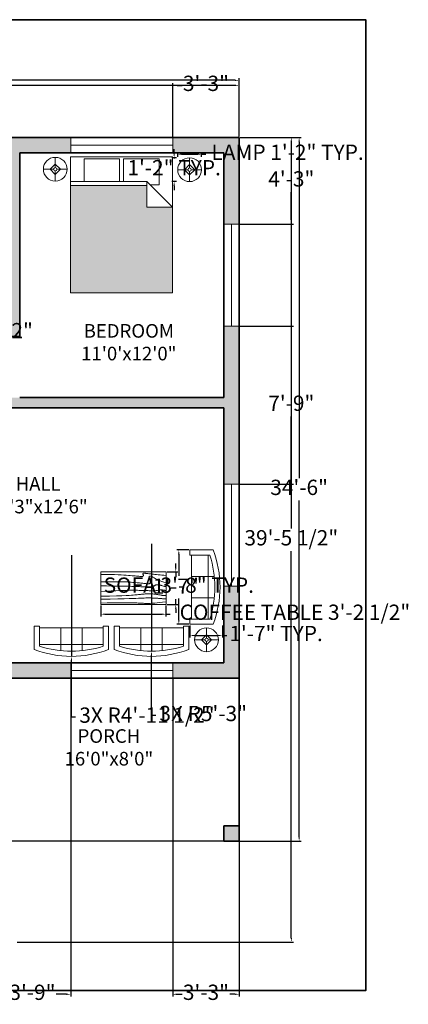
# Model space of a CAD drawing. Units: inches. Extents: x 1329 to 1989, y 1493 to 2072.
# Tile 4 of 4: x 1761 to 1989, y 1493 to 2072. Entities that reach past the tile are written whole.
import ezdxf

# ---------------------------------------------------------------- set-up
doc = ezdxf.new("R2010")
doc.units = ezdxf.units.IN
for name, color, linetype, lineweight in [('A-ANNO-DIMS', 2, 'Continuous', 18), ('A-ANNO-TTLB', 7, 'Continuous', 35), ('A-AREA-IDEN', 7, 'Continuous', 25), ('A-COLS', 7, 'Continuous', 35), ('A-FLOR', 7, 'Continuous', 25), ('A-FURN', 8, 'Continuous', 18), ('A-GLAZ', 4, 'Continuous', 18), ('A-WALL', 7, 'Continuous', 35)]:
    doc.layers.add(name, color=color, linetype=linetype, lineweight=lineweight)
for name, color, linetype, lineweight, true_color in [('A-COLS-PATT', 251, 'Continuous', 13, 0x636466), ('A-FURN-PATT', 18, 'Continuous', 13, 0x000000), ('A-WALL-PATT', 251, 'Continuous', 13, 0x636466)]:
    doc.layers.add(name, color=color, linetype=linetype, lineweight=lineweight, true_color=true_color)
doc.styles.get("Standard").update_dxf_attribs({"font": 'arial.ttf'})
doc.dimstyles.new('ISO-25', dxfattribs={"dimtxt": 9, "dimasz": 2.5, "dimexe": 1.25, "dimexo": 0.625, "dimgap": 2, "dimtad": 0, "dimtih": 1, "dimtoh": 1, "dimdec": 1, "dimlunit": 4, "dimtxsty": 'Standard', "dimcen": 2.5, "dimadec": 0, "dimazin": 0, "dimtfac": 0.5, "dimtdec": 1, "dimtmove": 0, "dimatfit": 3, "dimfxl": 1, "dimarcsym": 0})

# ---------------------------------------------------------------- blocks, each defined once
blk = doc.blocks.new('Bed - Queen')
for p, q in [((0, -80.00003), (0, 0)), ((0, 0), (59.99999, 0)), ((59.99999, 0), (59.99999, -80.00003)), ((7.99999, -1.2), (28.79998, -1.2)), ((7.99999, -14.4), (7.99999, -1.2)), ((28.79998, -1.2), (28.79998, -14.4)), ((31.19999, -1.2), (51.99999, -1.2)), ((31.19999, -14.4), (31.19999, -1.2)), ((51.99999, -1.2), (51.99999, -16.4)), ((0, -14.4), (44.8, -14.4)), ((44.8, -16.8), (0, -16.8)), ((59.99999, -29.6), (44.8, -14.4)), ((44.8, -14.4), (44.8, -29.6)), ((51.99999, -16.4), (46.79936, -16.4)), ((44.8, -29.6), (59.99999, -29.6)), ((59.99999, -80.00003), (0, -80.00003))]:
    blk.add_line(p, q)
blk = doc.blocks.new('Lamp - Table')
for p, q in [((0, 7), (0, 1)), ((-1, 0), (-7, 0)), ((0, 3), (-3, 0)), ((-3, 0), (0, -3)), ((3, 0), (0, 3)), ((0, -3), (3, 0)), ((1, 0), (7, 0)), ((0, -1), (0, -7))]:
    blk.add_line(p, q)
for radius in [7, 1]:
    blk.add_circle((0, 0), radius)
blk = doc.blocks.new('Sofa - Roundback 7 ft.')
for p, q in [((-12.00002, -32.4421), (-12.00003, -6.5971)), ((11.99997, -32.4421), (11.99998, -6.5971)), ((-36.000027, -34), (-36.000027, -11.4696)), ((-35.999844, -13.3819), (35.9998, -13.3819)), ((35.99998, -34), (35.99998, -11.4696)), ((-36.000027, -32.4421), (35.99998, -32.4421))]:
    blk.add_line(p, q)
for points in [[(-36.000027, -34), (-42.000027, -34), (-42.000027, -8)], [(41.99998, -8), (41.99998, -34), (35.99998, -34)]]:
    blk.add_lwpolyline(points)
for centre, radius, start, end in [((0, -114.25), 114.25, 68.43141, 111.5686), ((-0.00001, -127.1968), 121.1968, 72.72033, 107.2797)]:
    blk.add_arc(centre, radius, start, end)
blk = doc.blocks.new('Table - Rectangular Woodgrain 60 x 30 in.')
for p, q in [((0, 0), (0, -30)), ((60, 0), (0, 0)), ((60, -30), (60, 0)), ((0, -30), (60, -30))]:
    blk.add_line(p, q)
for points in [[(0, -2.4), (4.8155, -2.418), (9.0302, -2.4688), (12.709, -2.5477), (15.9167, -2.65), (18.7181, -2.7711), (21.1781, -2.9063), (23.3616, -3.0508), (25.3333, -3.2), (27.1477, -3.3495), (28.8172, -3.4958), (30.3437, -3.636), (31.7291, -3.7667), (32.9756, -3.8849), (34.0849, -3.9875), (35.059, -4.0714), (35.9, -4.1334), (36.6114, -4.1711), (37.2041, -4.1854), (37.6906, -4.1779), (38.0833, -4.15), (38.3948, -4.1034), (38.6375, -4.0396), (38.8239, -3.9602), (38.9666, -3.8667), (39.0764, -3.7608), (39.1573, -3.6448), (39.2116, -3.521), (39.2416, -3.3917), (39.2498, -3.2593), (39.2385, -3.1261), (39.21, -2.9944), (39.1666, -2.8667), (39.111, -2.7447), (39.0468, -2.6281), (38.978, -2.5163), (38.9083, -2.4083), (38.8418, -2.3035), (38.7823, -2.201), (38.7337, -2.1001), (38.7, -2), (38.6844, -1.9003), (38.6875, -1.8021), (38.7094, -1.707), (38.75, -1.6167), (38.8094, -1.5326), (38.8875, -1.4563), (38.9844, -1.3893), (39.1, -1.3333), (39.2351, -1.2896), (39.3937, -1.2583), (39.5804, -1.2396), (39.8, -1.2333), (40.057, -1.2396), (40.3562, -1.2583), (40.7023, -1.2896), (41.1, -1.3333), (41.5547, -1.3895), (42.0755, -1.4573), (42.6721, -1.5361), (43.3542, -1.625), (44.1316, -1.7233), (45.014, -1.8302), (46.0114, -1.9449), (47.1333, -2.0667), (48.3862, -2.1947), (49.7625, -2.3281), (51.2513, -2.4663), (52.8416, -2.6083), (54.5226, -2.7535), (56.2833, -2.9011), (58.1127, -3.0501), (60, -3.2)], [(0, -9.2), (6.5759, -9.0858), (11.9385, -9.0365), (16.2527, -9.0418), (19.6833, -9.0917), (22.3952, -9.1759), (24.5531, -9.2844), (26.322, -9.4069), (27.8666, -9.5333), (29.3241, -9.6553), (30.7203, -9.7719), (32.0532, -9.8837), (33.3208, -9.9917), (34.5213, -10.0965), (35.6526, -10.199), (36.7128, -10.2999), (37.7, -10.4), (38.6129, -10.4996), (39.4531, -10.5969), (40.223, -10.6895), (40.925, -10.775), (41.5613, -10.8512), (42.1344, -10.9156), (42.6465, -10.966), (43.1, -11), (43.4976, -11.0158), (43.8437, -11.0136), (44.143, -10.9942), (44.4, -10.9583), (44.6195, -10.9069), (44.8062, -10.8406), (44.9648, -10.7603), (45.1, -10.6667), (45.2155, -10.5598), (45.3114, -10.4365), (45.3871, -10.2929), (45.4416, -10.125), (45.4743, -9.929), (45.4844, -9.7011), (45.4709, -9.4371), (45.4333, -9.1333), (45.3716, -8.7883), (45.2896, -8.4104), (45.1919, -8.0107), (45.0833, -7.6), (44.9685, -7.1893), (44.8521, -6.7896), (44.7388, -6.4117), (44.6333, -6.0667), (44.54, -5.7628), (44.4614, -5.4979), (44.4001, -5.2675), (44.3583, -5.0667), (44.3384, -4.8909), (44.3427, -4.7354), (44.3736, -4.5956), (44.4333, -4.4667), (44.5236, -4.3453), (44.6427, -4.2333), (44.7884, -4.1339), (44.9583, -4.05), (45.1501, -3.9849), (45.3614, -3.9417), (45.59, -3.9234), (45.8333, -3.9333), (46.0915, -3.9749), (46.3734, -4.0531), (46.6906, -4.1736), (47.0542, -4.3417), (47.4756, -4.5629), (47.9661, -4.8427), (48.5372, -5.1866), (49.2, -5.6), (49.9676, -6.0844), (50.8594, -6.625), (51.8965, -7.2031), (53.1, -7.8), (54.491, -8.3969), (56.0906, -8.975), (57.9199, -9.5156), (60, -10)], [(0, -12.8), (5.1847, -12.9322), (9.6213, -13.0323), (13.3963, -13.1059), (16.5958, -13.1583), (19.3063, -13.1952), (21.614, -13.2219), (23.6054, -13.2439), (25.3666, -13.2667), (26.9728, -13.2947), (28.4531, -13.3281), (29.8256, -13.3663), (31.1083, -13.4083), (32.3191, -13.4535), (33.476, -13.501), (34.597, -13.5501), (35.7, -13.6), (36.7984, -13.6497), (37.8875, -13.6979), (38.9578, -13.743), (40, -13.7833), (41.0047, -13.8174), (41.9625, -13.8438), (42.864, -13.8607), (43.7, -13.8667), (44.4631, -13.8604), (45.1552, -13.8417), (45.7801, -13.8104), (46.3416, -13.7667), (46.8439, -13.7104), (47.2906, -13.6417), (47.6858, -13.5604), (48.0333, -13.4667), (48.3375, -13.3608), (48.6042, -13.2448), (48.8396, -13.121), (49.05, -12.9917), (49.2417, -12.8593), (49.4208, -12.7261), (49.5937, -12.5944), (49.7667, -12.4667), (49.9452, -12.3451), (50.1323, -12.2313), (50.3303, -12.1268), (50.5416, -12.0333), (50.7686, -11.9524), (51.0135, -11.8854), (51.2788, -11.8341), (51.5666, -11.8), (51.8785, -11.7843), (52.2116, -11.7865), (52.562, -11.8059), (52.926, -11.8417), (53.2998, -11.8931), (53.6795, -11.9594), (54.0614, -12.0397), (54.4416, -12.1333), (54.8223, -12.2401), (55.2293, -12.3625), (55.6942, -12.5037), (56.2489, -12.6667), (56.9251, -12.8547), (57.7545, -13.0708), (58.7689, -13.3182), (60, -13.6)], [(0, -18), (5.124, -17.7273), (9.6609, -17.5057), (13.6705, -17.3303), (17.2125, -17.1958), (20.3467, -17.0973), (23.1328, -17.0297), (25.6307, -16.9878), (27.9, -16.9667), (29.9928, -16.9617), (31.9302, -16.9703), (33.7254, -16.9907), (35.3917, -17.0208), (36.9423, -17.0588), (38.3906, -17.1026), (39.7499, -17.1503), (41.0333, -17.2), (42.2519, -17.2496), (43.4073, -17.2969), (44.4986, -17.3395), (45.525, -17.375), (46.4858, -17.4012), (47.3802, -17.4156), (48.2074, -17.416), (48.9667, -17.4), (49.6583, -17.3662), (50.2872, -17.3167), (50.8595, -17.2547), (51.3812, -17.1833), (51.8584, -17.1057), (52.2971, -17.025), (52.7034, -16.9443), (53.0833, -16.8667), (53.443, -16.7951), (53.789, -16.7313), (54.128, -16.6768), (54.4666, -16.6334), (54.8115, -16.6024), (55.1693, -16.5854), (55.5465, -16.5841), (55.95, -16.6), (56.3828, -16.6337), (56.8346, -16.6823), (57.2915, -16.7418), (57.7396, -16.8084), (58.165, -16.878), (58.5539, -16.9469), (58.8924, -17.0111), (59.1666, -17.0667), (59.3679, -17.1107), (59.5078, -17.1438), (59.6032, -17.1675), (59.6708, -17.1833), (59.7275, -17.193), (59.7901, -17.1979), (59.8753, -17.1998), (60, -17.2)], [(0, -22.4), (8.0098, -22.2501), (14.4094, -22.1011), (19.4168, -21.9535), (23.25, -21.8083), (26.1269, -21.6663), (28.2656, -21.5281), (29.884, -21.3947), (31.2, -21.2667), (32.3967, -21.1448), (33.5172, -21.0292), (34.5697, -20.9198), (35.5625, -20.8167), (36.5037, -20.7198), (37.4015, -20.6292), (38.2642, -20.5448), (39.1, -20.4667), (39.9164, -20.3951), (40.7187, -20.3313), (41.5117, -20.2768), (42.3, -20.2333), (43.0883, -20.2024), (43.8812, -20.1854), (44.6836, -20.1841), (45.5, -20.2), (46.3328, -20.234), (47.1747, -20.2844), (48.0163, -20.3488), (48.8479, -20.425), (49.66, -20.5106), (50.4429, -20.6031), (51.1872, -20.7004), (51.8833, -20.8), (52.5246, -20.8999), (53.1166, -20.9995), (53.6681, -21.0983), (54.1875, -21.1958), (54.6834, -21.2919), (55.1646, -21.3859), (55.6394, -21.4777), (56.1167, -21.5667), (56.6028, -21.6515), (57.0961, -21.7266), (57.5929, -21.7852), (58.0896, -21.8208), (58.5823, -21.8268), (59.0674, -21.7964), (59.5412, -21.723), (60, -21.6)], [(0, -25.2), (8.6355, -25.0504), (15.7026, -24.9031), (21.4049, -24.7606), (25.9458, -24.625), (29.529, -24.4988), (32.3578, -24.3844), (34.6359, -24.284), (36.5667, -24.2), (38.3213, -24.1341), (39.9417, -24.0854), (41.437, -24.0523), (42.8167, -24.0333), (44.0901, -24.0268), (45.2667, -24.0313), (46.3557, -24.0451), (47.3667, -24.0667), (48.309, -24.0947), (49.1928, -24.1287), (50.0284, -24.168), (50.826, -24.2125), (51.5959, -24.2617), (52.3483, -24.3151), (53.0935, -24.3725), (53.8417, -24.4334), (54.6009, -24.497), (55.3699, -24.561), (56.1454, -24.6226), (56.9239, -24.6792), (57.7021, -24.7279), (58.4764, -24.7662), (59.2435, -24.7911), (60, -24.8)], [(0, -28.8), (5.6867, -28.6681), (10.45, -28.5698), (14.407, -28.5012), (17.675, -28.4584), (20.3711, -28.4374), (22.6125, -28.4344), (24.5164, -28.4455), (26.2, -28.4667), (27.762, -28.4947), (29.2276, -28.5281), (30.6033, -28.5663), (31.8958, -28.6084), (33.1118, -28.6535), (34.2578, -28.7011), (35.3405, -28.7501), (36.3666, -28.8), (37.3443, -28.8497), (38.288, -28.8974), (39.2137, -28.9412), (40.1375, -28.9792), (41.0753, -29.0093), (42.0432, -29.0297), (43.0572, -29.0384), (44.1333, -29.0333), (45.2936, -29.0114), (46.5843, -28.9641), (48.0579, -28.8816), (49.7666, -28.7542), (51.7629, -28.5721), (54.0989, -28.3255), (56.8272, -28.0048), (60, -27.6)]]:
    blk.add_lwpolyline(points)
blk = doc.blocks.new('*D12')
at = {"layer": 'A-ANNO-DIMS', "color": 0, "lineweight": -2, "transparency": 16777216}
for p, q in [((1499.69, 2003.15), (1499.69, 2037.42)), ((1502.19, 2036.17), (1677.23, 2036.17)), ((1887.19, 2036.17), (1712.14, 2036.17)), ((1889.69, 2003.15), (1889.69, 2037.42))]:
    blk.add_line(p, q, dxfattribs=at)
at = {"layer": 'A-ANNO-DIMS', "color": 0, "transparency": 16777216}
for points in [[(1502.19, 2036.58), (1502.19, 2035.75), (1499.69, 2036.17)], [(1887.19, 2036.58), (1887.19, 2035.75), (1889.69, 2036.17)]]:
    blk.add_solid(points, dxfattribs=at)
at = {"layer": 'Defpoints', "color": 0, "transparency": 16777216}
for p in [(1889.69, 2036.17), (1499.69, 2002.52), (1889.69, 2002.52)]:
    blk.add_point(p, dxfattribs=at)
at = {"layer": 'A-ANNO-DIMS', "color": 0, "transparency": 16777216, "insert": (1694.69, 2036.17), "char_height": 9, "attachment_point": 5}
blk.add_mtext('32\'-6"', dxfattribs=at)
blk = doc.blocks.new('*D13')
at = {"layer": 'A-ANNO-DIMS', "color": 0, "lineweight": -2, "transparency": 16777216}
for p, q in [((1890.31, 2002.52), (1926.23, 2002.52)), ((1924.98, 2000.02), (1924.98, 1802.12)), ((1924.98, 1591.02), (1924.98, 1788.93)), ((1890.31, 1588.52), (1926.23, 1588.52))]:
    blk.add_line(p, q, dxfattribs=at)
at = {"layer": 'A-ANNO-DIMS', "color": 0, "transparency": 16777216}
for points in [[(1924.57, 2000.02), (1925.4, 2000.02), (1924.98, 2002.52)], [(1924.57, 1591.02), (1925.4, 1591.02), (1924.98, 1588.52)]]:
    blk.add_solid(points, dxfattribs=at)
at = {"layer": 'Defpoints', "color": 0, "transparency": 16777216}
for p in [(1889.69, 2002.52), (1889.69, 1588.52), (1924.98, 1588.52)]:
    blk.add_point(p, dxfattribs=at)
at = {"layer": 'A-ANNO-DIMS', "color": 0, "transparency": 16777216, "insert": (1924.98, 1795.52), "char_height": 9, "attachment_point": 5}
blk.add_mtext('34\'-6"', dxfattribs=at)
blk = doc.blocks.new('WIN-60IN')
for p, q in [((0, 0), (0, 9)), ((60, 0), (60, 9)), ((0, 4.5), (60, 4.5))]:
    blk.add_line(p, q)
blk = doc.blocks.new('*D21')
at = {"layer": 'A-ANNO-DIMS', "color": 0, "lineweight": -2, "transparency": 16777216}
for p, q in [((1853.58, 1991.21), (1853.58, 1993.94)), ((1867.58, 1991.21), (1867.58, 1993.94)), ((1856.08, 1992.69), (1865.08, 1992.69)), ((1867.58, 1992.69), (1870.08, 1992.69))]:
    blk.add_line(p, q, dxfattribs=at)
at = {"layer": 'A-ANNO-DIMS', "color": 0, "transparency": 16777216}
for points in [[(1856.08, 1993.1), (1856.08, 1992.27), (1853.58, 1992.69)], [(1865.08, 1993.1), (1865.08, 1992.27), (1867.58, 1992.69)]]:
    blk.add_solid(points, dxfattribs=at)
at = {"layer": 'Defpoints', "color": 0, "transparency": 16777216}
for p in [(1853.58, 1990.59), (1867.58, 1992.69), (1867.58, 1990.59)]:
    blk.add_point(p, dxfattribs=at)
at = {"layer": 'A-ANNO-DIMS', "color": 0, "transparency": 16777216, "insert": (1918.18, 1992.69), "char_height": 9, "attachment_point": 5}
blk.add_mtext('LAMP 1\'-2" TYP.', dxfattribs=at)
blk = doc.blocks.new('*D22')
at = {"layer": 'A-ANNO-DIMS', "color": 0, "lineweight": -2, "transparency": 16777216}
for p, q in [((1851.48, 1993.09), (1851.48, 1995.59)), ((1852.96, 1990.59), (1850.23, 1990.59)), ((1851.48, 1990.59), (1851.48, 1990.11)), ((1852.96, 1976.59), (1850.23, 1976.59)), ((1851.48, 1976.59), (1851.48, 1977.06)), ((1851.48, 1974.09), (1851.48, 1971.59))]:
    blk.add_line(p, q, dxfattribs=at)
at = {"layer": 'A-ANNO-DIMS', "color": 0, "transparency": 16777216}
for points in [[(1851.07, 1993.09), (1851.9, 1993.09), (1851.48, 1990.59)], [(1851.07, 1974.09), (1851.9, 1974.09), (1851.48, 1976.59)]]:
    blk.add_solid(points, dxfattribs=at)
at = {"layer": 'Defpoints', "color": 0, "transparency": 16777216}
for p in [(1851.48, 1990.59), (1853.58, 1990.59), (1853.58, 1976.59)]:
    blk.add_point(p, dxfattribs=at)
at = {"layer": 'A-ANNO-DIMS', "color": 0, "transparency": 16777216, "insert": (1851.48, 1983.59), "char_height": 9, "attachment_point": 5}
blk.add_mtext('1\'-2" TYP.', dxfattribs=at)
blk = doc.blocks.new('*D25')
at = {"layer": 'A-ANNO-DIMS', "color": 0, "lineweight": -2, "transparency": 16777216}
for p, q in [((1860.18, 1759.87), (1852.99, 1759.87)), ((1854.24, 1757.37), (1854.24, 1744.65)), ((1854.24, 1718.61), (1854.24, 1731.33)), ((1860.18, 1716.11), (1852.99, 1716.11))]:
    blk.add_line(p, q, dxfattribs=at)
at = {"layer": 'A-ANNO-DIMS', "color": 0, "transparency": 16777216}
for points in [[(1853.82, 1757.37), (1854.65, 1757.37), (1854.24, 1759.87)], [(1853.82, 1718.61), (1854.65, 1718.61), (1854.24, 1716.11)]]:
    blk.add_solid(points, dxfattribs=at)
at = {"layer": 'Defpoints', "color": 0, "transparency": 16777216}
for p in [(1860.8, 1759.87), (1854.24, 1716.11), (1860.8, 1716.11)]:
    blk.add_point(p, dxfattribs=at)
at = {"layer": 'A-ANNO-DIMS', "color": 0, "transparency": 16777216, "insert": (1854.24, 1737.99), "char_height": 9, "attachment_point": 5}
blk.add_mtext('SOFA 3\'-8" TYP.', dxfattribs=at)
blk = doc.blocks.new('*D26')
at = {"layer": 'A-ANNO-DIMS', "color": 0, "lineweight": -2, "transparency": 16777216}
for p, q in [((1860.8, 1715.49), (1860.8, 1708.3)), ((1879.9, 1715.49), (1879.9, 1708.3)), ((1863.3, 1709.55), (1877.4, 1709.55)), ((1879.9, 1709.55), (1882.4, 1709.55))]:
    blk.add_line(p, q, dxfattribs=at)
at = {"layer": 'A-ANNO-DIMS', "color": 0, "transparency": 16777216}
for points in [[(1863.3, 1709.96), (1863.3, 1709.13), (1860.8, 1709.55)], [(1877.4, 1709.96), (1877.4, 1709.13), (1879.9, 1709.55)]]:
    blk.add_solid(points, dxfattribs=at)
at = {"layer": 'Defpoints', "color": 0, "transparency": 16777216}
for p in [(1860.8, 1716.11), (1879.9, 1716.11), (1879.9, 1709.55)]:
    blk.add_point(p, dxfattribs=at)
at = {"layer": 'A-ANNO-DIMS', "color": 0, "transparency": 16777216, "insert": (1911.41, 1709.55), "char_height": 9, "attachment_point": 5}
blk.add_mtext('1\'-7" TYP.', dxfattribs=at)
blk = doc.blocks.new('*D29')
at = {"layer": 'A-ANNO-DIMS', "color": 0, "lineweight": -2, "transparency": 16777216}
for p, q in [((1661.14, 1889.61), (1661.14, 1886.47)), ((1677.89, 1889.61), (1677.89, 1886.47)), ((1663.64, 1887.72), (1675.39, 1887.72)), ((1677.89, 1887.72), (1680.39, 1887.72))]:
    blk.add_line(p, q, dxfattribs=at)
at = {"layer": 'A-ANNO-DIMS', "color": 0, "transparency": 16777216}
for points in [[(1663.64, 1888.14), (1663.64, 1887.31), (1661.14, 1887.72)], [(1675.39, 1888.14), (1675.39, 1887.31), (1677.89, 1887.72)]]:
    blk.add_solid(points, dxfattribs=at)
at = {"layer": 'Defpoints', "color": 0, "transparency": 16777216}
for p in [(1661.14, 1890.24), (1677.89, 1890.24), (1677.89, 1887.72)]:
    blk.add_point(p, dxfattribs=at)
at = {"layer": 'A-ANNO-DIMS', "color": 0, "transparency": 16777216, "insert": (1725.25, 1887.72), "char_height": 9, "attachment_point": 5}
blk.add_mtext('BASIN 1\'-4 1/2"', dxfattribs=at)
blk = doc.blocks.new('*D35')
at = {"layer": 'A-ANNO-DIMS', "color": 0, "lineweight": -2, "transparency": 16777216}
for p, q in [((1808.39, 1727.17), (1808.39, 1720.8)), ((1846.7, 1727.17), (1846.7, 1720.8)), ((1810.89, 1722.05), (1844.2, 1722.05)), ((1846.7, 1722.05), (1849.2, 1722.05))]:
    blk.add_line(p, q, dxfattribs=at)
at = {"layer": 'A-ANNO-DIMS', "color": 0, "transparency": 16777216}
for points in [[(1810.89, 1722.47), (1810.89, 1721.64), (1808.39, 1722.05)], [(1844.2, 1722.47), (1844.2, 1721.64), (1846.7, 1722.05)]]:
    blk.add_solid(points, dxfattribs=at)
at = {"layer": 'Defpoints', "color": 0, "transparency": 16777216}
for p in [(1808.39, 1727.8), (1846.7, 1727.8), (1846.7, 1722.05)]:
    blk.add_point(p, dxfattribs=at)
at = {"layer": 'A-ANNO-DIMS', "color": 0, "transparency": 16777216, "insert": (1922.5, 1722.05), "char_height": 9, "attachment_point": 5}
blk.add_mtext('COFFEE TABLE 3\'-2 1/2"', dxfattribs=at)
blk = doc.blocks.new('*D36')
at = {"layer": 'A-ANNO-DIMS', "color": 0, "lineweight": -2, "transparency": 16777216}
for p, q in [((1852.45, 1749.46), (1852.45, 1751.96)), ((1847.32, 1746.96), (1853.7, 1746.96)), ((1852.45, 1746.96), (1852.45, 1743.9)), ((1847.32, 1727.8), (1853.7, 1727.8)), ((1852.45, 1727.8), (1852.45, 1730.86)), ((1852.45, 1725.3), (1852.45, 1722.8))]:
    blk.add_line(p, q, dxfattribs=at)
at = {"layer": 'A-ANNO-DIMS', "color": 0, "transparency": 16777216}
for points in [[(1852.03, 1749.46), (1852.86, 1749.46), (1852.45, 1746.96)], [(1852.03, 1725.3), (1852.86, 1725.3), (1852.45, 1727.8)]]:
    blk.add_solid(points, dxfattribs=at)
at = {"layer": 'Defpoints', "color": 0, "transparency": 16777216}
for p in [(1846.7, 1746.96), (1852.45, 1746.96), (1846.7, 1727.8)]:
    blk.add_point(p, dxfattribs=at)
at = {"layer": 'A-ANNO-DIMS', "color": 0, "transparency": 16777216, "insert": (1852.45, 1737.38), "char_height": 9, "attachment_point": 5}
blk.add_mtext('1\'-7"', dxfattribs=at)
blk = doc.blocks.new('*D37')
at = {"layer": 'A-ANNO-DIMS', "color": 0, "lineweight": -2, "transparency": 16777216}
for p, q in [((1406.14, 1850.15), (1406.14, 2034.47)), ((1889.69, 2003.15), (1889.69, 2034.47)), ((1408.64, 2033.22), (1619.79, 2033.22)), ((1887.19, 2033.22), (1676.04, 2033.22))]:
    blk.add_line(p, q, dxfattribs=at)
at = {"layer": 'A-ANNO-DIMS', "color": 0, "transparency": 16777216}
for points in [[(1408.64, 2033.64), (1408.64, 2032.81), (1406.14, 2033.22)], [(1887.19, 2033.64), (1887.19, 2032.81), (1889.69, 2033.22)]]:
    blk.add_solid(points, dxfattribs=at)
at = {"layer": 'Defpoints', "color": 0, "transparency": 16777216}
for p in [(1889.69, 2033.22), (1889.69, 2002.52), (1406.14, 1849.52)]:
    blk.add_point(p, dxfattribs=at)
at = {"layer": 'A-ANNO-DIMS', "color": 0, "transparency": 16777216, "insert": (1647.91, 2033.22), "char_height": 9, "attachment_point": 5}
blk.add_mtext('40\'-3 1/2"', dxfattribs=at)
blk = doc.blocks.new('*D38')
at = {"layer": 'A-ANNO-DIMS', "color": 0, "lineweight": -2, "transparency": 16777216}
for p, q in [((1890.31, 2002.52), (1921.64, 2002.52)), ((1920.39, 2000.02), (1920.39, 1772.49)), ((1920.39, 1531.65), (1920.39, 1759.18)), ((1759.27, 1529.15), (1921.64, 1529.15))]:
    blk.add_line(p, q, dxfattribs=at)
at = {"layer": 'A-ANNO-DIMS', "color": 0, "transparency": 16777216}
for points in [[(1919.97, 2000.02), (1920.8, 2000.02), (1920.39, 2002.52)], [(1919.97, 1531.65), (1920.8, 1531.65), (1920.39, 1529.15)]]:
    blk.add_solid(points, dxfattribs=at)
at = {"layer": 'Defpoints', "color": 0, "transparency": 16777216}
for p in [(1889.69, 2002.52), (1758.64, 1529.15), (1920.39, 1529.15)]:
    blk.add_point(p, dxfattribs=at)
at = {"layer": 'A-ANNO-DIMS', "color": 0, "transparency": 16777216, "insert": (1920.39, 1765.84), "char_height": 9, "attachment_point": 5}
blk.add_mtext('39\'-5 1/2"', dxfattribs=at)
blk = doc.blocks.new('*D42')
at = {"layer": 'A-ANNO-DIMS', "color": 0, "lineweight": -2, "transparency": 16777216}
for p, q in [((1850.69, 2003.15), (1850.69, 2034.47)), ((1889.69, 2003.15), (1889.69, 2034.47)), ((1853.19, 2033.22), (1856.23, 2033.22)), ((1887.19, 2033.22), (1884.15, 2033.22))]:
    blk.add_line(p, q, dxfattribs=at)
at = {"layer": 'A-ANNO-DIMS', "color": 0, "transparency": 16777216}
for points in [[(1853.19, 2033.64), (1853.19, 2032.81), (1850.69, 2033.22)], [(1887.19, 2033.64), (1887.19, 2032.81), (1889.69, 2033.22)]]:
    blk.add_solid(points, dxfattribs=at)
at = {"layer": 'Defpoints', "color": 0, "transparency": 16777216}
for p in [(1889.69, 2033.22), (1850.69, 2002.52), (1889.69, 2002.52)]:
    blk.add_point(p, dxfattribs=at)
at = {"layer": 'A-ANNO-DIMS', "color": 0, "transparency": 16777216, "insert": (1870.19, 2033.22), "char_height": 9, "attachment_point": 5}
blk.add_mtext('3\'-3"', dxfattribs=at)
blk = doc.blocks.new('*D43')
at = {"layer": 'A-ANNO-DIMS', "color": 0, "lineweight": -2, "transparency": 16777216}
for p, q in [((1890.31, 1891.52), (1921.64, 1891.52)), ((1920.39, 1889.02), (1920.39, 1851.62)), ((1920.39, 1801.02), (1920.39, 1838.43)), ((1890.31, 1798.52), (1921.64, 1798.52))]:
    blk.add_line(p, q, dxfattribs=at)
at = {"layer": 'A-ANNO-DIMS', "color": 0, "transparency": 16777216}
for points in [[(1919.97, 1889.02), (1920.8, 1889.02), (1920.39, 1891.52)], [(1919.97, 1801.02), (1920.8, 1801.02), (1920.39, 1798.52)]]:
    blk.add_solid(points, dxfattribs=at)
at = {"layer": 'Defpoints', "color": 0, "transparency": 16777216}
for p in [(1889.69, 1891.52), (1889.69, 1798.52), (1920.39, 1798.52)]:
    blk.add_point(p, dxfattribs=at)
at = {"layer": 'A-ANNO-DIMS', "color": 0, "transparency": 16777216, "insert": (1920.39, 1845.02), "char_height": 9, "attachment_point": 5}
blk.add_mtext('7\'-9"', dxfattribs=at)
blk = doc.blocks.new('*D44')
at = {"layer": 'A-ANNO-DIMS', "color": 0, "lineweight": -2, "transparency": 16777216}
for p, q in [((1890.31, 2002.52), (1921.64, 2002.52)), ((1920.39, 2000.02), (1920.39, 1983.62)), ((1920.39, 1954.02), (1920.39, 1970.43)), ((1890.31, 1951.52), (1921.64, 1951.52))]:
    blk.add_line(p, q, dxfattribs=at)
at = {"layer": 'A-ANNO-DIMS', "color": 0, "transparency": 16777216}
for points in [[(1919.97, 2000.02), (1920.8, 2000.02), (1920.39, 2002.52)], [(1919.97, 1954.02), (1920.8, 1954.02), (1920.39, 1951.52)]]:
    blk.add_solid(points, dxfattribs=at)
at = {"layer": 'Defpoints', "color": 0, "transparency": 16777216}
for p in [(1889.69, 2002.52), (1920.39, 2002.52), (1889.69, 1951.52)]:
    blk.add_point(p, dxfattribs=at)
at = {"layer": 'A-ANNO-DIMS', "color": 0, "transparency": 16777216, "insert": (1920.39, 1977.02), "char_height": 9, "attachment_point": 5}
blk.add_mtext('4\'-3"', dxfattribs=at)
blk = doc.blocks.new('*D54')
at = {"layer": 'A-ANNO-DIMS', "color": 0, "lineweight": -2, "transparency": 16777216}
for p, q in [((1745.69, 1683.9), (1745.69, 1497.2)), ((1790.69, 1683.9), (1790.69, 1497.2)), ((1748.19, 1498.45), (1754.23, 1498.45)), ((1788.19, 1498.45), (1782.15, 1498.45))]:
    blk.add_line(p, q, dxfattribs=at)
at = {"layer": 'A-ANNO-DIMS', "color": 0, "transparency": 16777216}
for points in [[(1748.19, 1498.87), (1748.19, 1498.03), (1745.69, 1498.45)], [(1788.19, 1498.87), (1788.19, 1498.03), (1790.69, 1498.45)]]:
    blk.add_solid(points, dxfattribs=at)
at = {"layer": 'Defpoints', "color": 0, "transparency": 16777216}
for p in [(1745.69, 1684.52), (1790.69, 1684.52), (1790.69, 1498.45)]:
    blk.add_point(p, dxfattribs=at)
at = {"layer": 'A-ANNO-DIMS', "color": 0, "transparency": 16777216, "insert": (1768.19, 1498.45), "char_height": 9, "attachment_point": 5}
blk.add_mtext('3\'-9"', dxfattribs=at)
blk = doc.blocks.new('*D55')
at = {"layer": 'A-ANNO-DIMS', "color": 0, "lineweight": -2, "transparency": 16777216}
for p, q in [((1850.69, 1683.9), (1850.69, 1497.2)), ((1889.69, 1683.9), (1889.69, 1497.2)), ((1853.19, 1498.45), (1856.23, 1498.45)), ((1887.19, 1498.45), (1884.15, 1498.45))]:
    blk.add_line(p, q, dxfattribs=at)
at = {"layer": 'A-ANNO-DIMS', "color": 0, "transparency": 16777216}
for points in [[(1853.19, 1498.87), (1853.19, 1498.03), (1850.69, 1498.45)], [(1887.19, 1498.87), (1887.19, 1498.03), (1889.69, 1498.45)]]:
    blk.add_solid(points, dxfattribs=at)
at = {"layer": 'Defpoints', "color": 0, "transparency": 16777216}
for p in [(1850.69, 1684.52), (1889.69, 1684.52), (1889.69, 1498.45)]:
    blk.add_point(p, dxfattribs=at)
at = {"layer": 'A-ANNO-DIMS', "color": 0, "transparency": 16777216, "insert": (1870.19, 1498.45), "char_height": 9, "attachment_point": 5}
blk.add_mtext('3\'-3"', dxfattribs=at)
blk = doc.blocks.new('*D56')
at = {"layer": 'A-ANNO-DIMS', "color": 0, "lineweight": -2, "transparency": 16777216}
for p, q in [((1838.16, 1763.48), (1838.16, 1700.35)), ((1838.16, 1662.47), (1838.16, 1697.85)), ((1840.66, 1662.47), (1838.16, 1662.47))]:
    blk.add_line(p, q, dxfattribs=at)
at = {"layer": 'A-ANNO-DIMS', "color": 0, "transparency": 16777216}
blk.add_solid([(1838.58, 1697.85), (1837.74, 1697.85), (1838.16, 1700.35)], dxfattribs=at)
at = {"layer": 'Defpoints', "color": 0, "transparency": 16777216}
for p in [(1838.16, 1763.48), (1838.16, 1700.35)]:
    blk.add_point(p, dxfattribs=at)
at = {"layer": 'A-ANNO-DIMS', "color": 0, "transparency": 16777216, "insert": (1868.6, 1662.47), "char_height": 9, "attachment_point": 5}
blk.add_mtext('3X R5\'-3"', dxfattribs=at)
blk = doc.blocks.new('*D57')
at = {"layer": 'A-ANNO-DIMS', "color": 0, "lineweight": -2, "transparency": 16777216}
for p, q in [((1791.08, 1756.74), (1791.08, 1697.22)), ((1791.08, 1661.51), (1791.08, 1694.72)), ((1793.58, 1661.51), (1791.08, 1661.51))]:
    blk.add_line(p, q, dxfattribs=at)
at = {"layer": 'A-ANNO-DIMS', "color": 0, "transparency": 16777216}
blk.add_solid([(1791.5, 1694.72), (1790.67, 1694.72), (1791.08, 1697.22)], dxfattribs=at)
at = {"layer": 'Defpoints', "color": 0, "transparency": 16777216}
for p in [(1791.08, 1756.74), (1791.08, 1697.22)]:
    blk.add_point(p, dxfattribs=at)
at = {"layer": 'A-ANNO-DIMS', "color": 0, "transparency": 16777216, "insert": (1835.5, 1661.51), "char_height": 9, "attachment_point": 5}
blk.add_mtext('3X R4\'-11 1/2"', dxfattribs=at)

msp = doc.modelspace()

# ---------------------------------------------------------------- hatches: boundary and pattern name
at = {"layer": 'A-COLS-PATT'}
h = msp.add_hatch(color=256, dxfattribs=at)
h.dxf.hatch_style = 1
h.paths.add_polyline_path([(1889.69, 1597.52), (1880.69, 1597.52), (1880.69, 1588.52), (1889.69, 1588.52)])
at = {"layer": 'A-FURN-PATT'}
h = msp.add_hatch(color=256, dxfattribs=at)
h.dxf.hatch_style = 1
h.paths.add_polyline_path([(1610.17, 1960.57), (1594.97, 1960.57), (1594.97, 1973.37), (1550.17, 1973.37), (1550.17, 1910.17), (1610.17, 1910.17)])
h.paths.add_polyline_path([(1850.61, 1961.54), (1835.41, 1961.54), (1835.41, 1974.34), (1790.61, 1974.34), (1790.61, 1911.14), (1850.61, 1911.14)])
at = {"layer": 'A-WALL-PATT'}
h = msp.add_hatch(color=256, dxfattribs=at)
h.dxf.hatch_style = 1
h.paths.add_polyline_path([(1550.69, 2002.52), (1499.69, 2002.52), (1499.69, 1951.52), (1508.69, 1951.52), (1508.69, 1993.52), (1550.69, 1993.52)])
h.paths.add_polyline_path([(1670.69, 2002.52), (1610.69, 2002.52), (1610.69, 1993.52), (1652.69, 1993.52), (1652.69, 1885.52), (1658.69, 1885.52), (1658.69, 1903.52), (1706.69, 1903.52), (1712.69, 1903.52), (1712.69, 1909.52), (1706.69, 1909.52), (1658.69, 1909.52), (1658.69, 1993.52), (1670.69, 1993.52)])
h.paths.add_polyline_path([(1721.69, 2002.52), (1694.69, 2002.52), (1694.69, 1993.52), (1706.69, 1993.52), (1706.69, 1939.52), (1712.69, 1939.52), (1730.69, 1939.52), (1730.69, 1945.52), (1712.69, 1945.52), (1712.69, 1993.52), (1721.69, 1993.52)])
h.paths.add_polyline_path([(1790.69, 2002.52), (1745.69, 2002.52), (1745.69, 1993.52), (1754.69, 1993.52), (1754.69, 1945.52), (1754.69, 1939.52), (1754.69, 1885.52), (1760.69, 1885.52), (1760.69, 1993.52), (1790.69, 1993.52)])
h.paths.add_polyline_path([(1889.69, 2002.52), (1850.69, 2002.52), (1850.69, 1993.52), (1880.69, 1993.52), (1880.69, 1951.52), (1889.69, 1951.52)])
h.paths.add_polyline_path([(1889.69, 1891.52), (1880.69, 1891.52), (1880.69, 1849.52), (1760.69, 1849.52), (1754.69, 1849.52), (1688.69, 1849.52), (1688.69, 1843.52), (1697.69, 1843.52), (1760.69, 1843.52), (1880.69, 1843.52), (1880.69, 1798.52), (1889.69, 1798.52)])
h.paths.add_polyline_path([(1658.69, 1849.52), (1652.69, 1849.52), (1508.69, 1849.52), (1508.69, 1891.52), (1499.69, 1891.52), (1499.69, 1849.52), (1406.14, 1849.52), (1406.14, 1828.52), (1415.14, 1828.52), (1415.14, 1840.52), (1508.69, 1840.52), (1652.69, 1840.52), (1658.69, 1840.52)])
h.paths.add_polyline_path([(1658.69, 1804.52), (1652.69, 1804.52), (1652.69, 1768.52), (1508.69, 1768.52), (1415.14, 1768.52), (1415.14, 1780.52), (1406.14, 1780.52), (1406.14, 1759.52), (1499.69, 1759.52), (1499.69, 1709.88), (1508.69, 1709.88), (1508.69, 1759.52), (1658.69, 1759.52)])
h.paths.add_polyline_path([(1508.69, 1649.88), (1499.69, 1649.88), (1499.69, 1618.52), (1568.69, 1618.52), (1568.69, 1627.52), (1508.69, 1627.52)])
h.paths.add_polyline_path([(1697.69, 1684.52), (1697.69, 1693.52), (1697.69, 1795.52), (1688.69, 1795.52), (1688.69, 1693.52), (1688.69, 1684.52), (1688.69, 1627.52), (1628.69, 1627.52), (1628.69, 1618.52), (1688.69, 1618.52), (1688.69, 1588.52), (1697.69, 1588.52), (1697.69, 1618.52)])
h.paths.add_polyline_path([(1790.69, 1693.52), (1760.69, 1693.52), (1745.69, 1693.52), (1745.69, 1684.52), (1760.69, 1684.52), (1790.69, 1684.52)])
h.paths.add_polyline_path([(1889.69, 1738.52), (1880.69, 1738.52), (1880.69, 1693.52), (1850.69, 1693.52), (1850.69, 1684.52), (1880.69, 1684.52), (1889.69, 1684.52)])

# ---------------------------------------------------------------- linework, layer by layer
at = {"layer": 'A-ANNO-TTLB'}
msp.add_lwpolyline([(1329.11, 2071.84), (1964.17, 2071.84), (1964.17, 1500.65), (1329.11, 1500.65)], close=True, dxfattribs=at)
at = {"layer": 'A-COLS'}
for p, q in [((1880.69, 1597.52), (1889.69, 1597.52)), ((1880.69, 1597.52), (1880.69, 1588.52)), ((1880.69, 1588.52), (1889.69, 1588.52))]:
    msp.add_line(p, q, dxfattribs=at)
at = {"layer": 'A-FLOR'}
msp.add_line((1889.69, 1588.52), (1697.69, 1588.52), dxfattribs=at)
at = {"layer": 'A-WALL'}
for p, q in [((1499.69, 2002.52), (1889.69, 2002.52)), ((1889.69, 2002.52), (1889.69, 1588.52)), ((1760.69, 1993.52), (1760.69, 1885.52)), ((1760.69, 1993.52), (1880.69, 1993.52)), ((1880.69, 1993.52), (1880.69, 1849.52)), ((1754.69, 1885.52), (1760.69, 1885.52)), ((1760.69, 1849.52), (1880.69, 1849.52)), ((1760.69, 1843.52), (1697.69, 1843.52)), ((1760.69, 1843.52), (1880.69, 1843.52)), ((1880.69, 1843.52), (1880.69, 1693.52)), ((1760.69, 1693.52), (1745.69, 1693.52)), ((1760.69, 1693.52), (1880.69, 1693.52)), ((1760.69, 1684.52), (1745.69, 1684.52)), ((1760.69, 1684.52), (1880.69, 1684.52)), ((1880.69, 1684.52), (1889.69, 1684.52))]:
    msp.add_line(p, q, dxfattribs=at)

# ---------------------------------------------------------------- block references
at = {"layer": 'A-FURN'}
for name, p in [('Lamp - Table', (1781.61, 1983.85)), ('Bed - Queen', (1790.61, 1991.14)), ('Lamp - Table', (1860.58, 1983.59)), ('Lamp - Table', (1870.55, 1707.01))]:
    msp.add_blockref(name, p, dxfattribs=at)
at = {"layer": 'A-FURN', "xscale": 0.5209331790706359, "yscale": 0.5209331790706359, "zscale": 0.5209331790706359}
for p, rotation in [((1878.51, 1737.99), 270), ((1791.08, 1697.22), 180), ((1838.16, 1697.22), 180)]:
    msp.add_blockref('Sofa - Roundback 7 ft.', p, dxfattribs=dict(at, rotation=rotation))
at = {"layer": 'A-FURN', "xscale": 0.6385557700590637, "yscale": 0.6385557700590637, "zscale": 0.6385557700590637}
msp.add_blockref('Table - Rectangular Woodgrain 60 x 30 in.', (1808.39, 1746.96), dxfattribs=at)
at = {"layer": 'A-GLAZ'}
msp.add_blockref('WIN-60IN', (1790.69, 1993.52), dxfattribs=at)
for p, rotation in [((1880.69, 1951.52), 269.9999999999997), ((1880.69, 1798.52), 270.000000000001), ((1850.69, 1693.52), 180)]:
    msp.add_blockref('WIN-60IN', p, dxfattribs=dict(at, rotation=rotation))

# ---------------------------------------------------------------- texts
at = {"layer": 'A-AREA-IDEN', "char_height": 8, "attachment_point": 1}
for s, width, insert in [('\\pxqc;{\\fArial|b1|i0|c0|p34;BEDROOM\\P11\'0\'x12\'0"}', 94.8064, (1777.44, 1892.76)), ('\\pxqc;{\\fArial|b1|i0|c0|p34;HALL\\P15\'3"x12\'6"}', 85.2875, (1728.9, 1802.74)), ('\\pxqc;{\\fArial|b1|i0|c0|p34;PORCH\\P16\'0"x8\'0"}', 90.4304, (1767.92, 1654.38))]:
    msp.add_mtext_dynamic_manual_height_columns(s, width=width, gutter_width=12.5, heights=[0], dxfattribs=dict(at, insert=insert))

# ---------------------------------------------------------------- dimensions: what is measured, and where the dimension line sits
at = {"layer": 'A-ANNO-DIMS'}
for base, p1, p2, override, picture, middle in [((1889.6864, 2033.2237), (1406.141, 1849.5237), (1889.6864, 2002.5237), {"dimdec": 1, "dimlfac": 1, "dimrnd": 0, "dimzin": 1, "dimdsep": 46, "dimlunit": 4, "dimfrac": 2}, '*D37', (1647.9137, 2033.2237)), ((1889.69, 2036.17), (1499.69, 2002.52), (1889.69, 2002.52), {"dimclrd": 0, "dimclre": 0, "dimclrt": 0}, '*D12', (1694.69, 2036.17)), ((1889.69, 2033.22), (1850.69, 2002.52), (1889.69, 2002.52), {"dimdec": 1, "dimlfac": 1, "dimrnd": 0, "dimzin": 1, "dimdsep": 46, "dimlunit": 4, "dimfrac": 2}, '*D42', (1870.19, 2033.22)), ((1790.69, 1498.45), (1745.69, 1684.52), (1790.69, 1684.52), {"dimdec": 1, "dimlfac": 1, "dimrnd": 0, "dimzin": 1, "dimdsep": 46, "dimlunit": 4, "dimfrac": 2}, '*D54', (1768.19, 1498.45)), ((1889.69, 1498.45), (1850.69, 1684.52), (1889.69, 1684.52), {"dimdec": 1, "dimlfac": 1, "dimrnd": 0, "dimzin": 1, "dimdsep": 46, "dimlunit": 4, "dimfrac": 2}, '*D55', (1870.19, 1498.45))]:
    dim = msp.add_linear_dim(base=base, p1=p1, p2=p2, dimstyle='ISO-25', override=override, dxfattribs=at)
    dim.commit()
    dim.dimension.update_dxf_attribs({"geometry": picture, "text_midpoint": middle})
for base, p1, p2, text, picture, middle in [((1867.58, 1992.69), (1853.58, 1990.59), (1867.58, 1990.59), 'LAMP <> TYP.', '*D21', (1918.18, 1992.69)), ((1677.8867, 1887.7233), (1661.1398, 1890.2354), (1677.8867, 1890.2354), 'BASIN <>', '*D29', (1725.2472, 1887.7233)), ((1846.7, 1722.05), (1808.39, 1727.8), (1846.7, 1727.8), 'COFFEE TABLE <>', '*D35', (1922.5, 1722.05)), ((1879.9, 1709.55), (1860.8, 1716.11), (1879.9, 1716.11), '<> TYP.', '*D26', (1911.41, 1709.55))]:
    dim = msp.add_linear_dim(base=base, p1=p1, p2=p2, text=text, dimstyle='ISO-25', override={"dimdec": 1, "dimlfac": 1, "dimrnd": 0, "dimzin": 1, "dimdsep": 46, "dimlunit": 4, "dimfrac": 2}, dxfattribs=at)
    dim.commit()
    dim.dimension.update_dxf_attribs({"geometry": picture, "text_midpoint": middle})
for base, p1, p2, override, picture, middle in [((1920.39, 1529.15), (1889.69, 2002.52), (1758.64, 1529.15), {"dimdec": 1, "dimlfac": 1, "dimrnd": 0, "dimzin": 1, "dimdsep": 46, "dimlunit": 4, "dimfrac": 2}, '*D38', (1920.39, 1765.84)), ((1924.98, 1588.52), (1889.69, 2002.52), (1889.69, 1588.52), {"dimclrd": 0, "dimclre": 0, "dimclrt": 0}, '*D13', (1924.98, 1795.52)), ((1920.39, 2002.52), (1889.69, 1951.52), (1889.69, 2002.52), {"dimdec": 1, "dimlfac": 1, "dimrnd": 0, "dimzin": 1, "dimdsep": 46, "dimlunit": 4, "dimfrac": 2}, '*D44', (1920.39, 1977.02)), ((1920.39, 1798.52), (1889.69, 1891.52), (1889.69, 1798.52), {"dimdec": 1, "dimlfac": 1, "dimrnd": 0, "dimzin": 1, "dimdsep": 46, "dimlunit": 4, "dimfrac": 2}, '*D43', (1920.39, 1845.02)), ((1852.45, 1746.96), (1846.7, 1727.8), (1846.7, 1746.96), {"dimdec": 1, "dimlfac": 1, "dimrnd": 0, "dimzin": 1, "dimdsep": 46, "dimlunit": 4, "dimfrac": 2}, '*D36', (1852.45, 1737.38))]:
    dim = msp.add_linear_dim(base=base, p1=p1, p2=p2, angle=90, dimstyle='ISO-25', override=override, dxfattribs=at)
    dim.commit()
    dim.dimension.update_dxf_attribs({"geometry": picture, "text_midpoint": middle})
for base, p1, p2, angle, text, picture, middle in [((1851.48, 1990.59), (1853.58, 1976.59), (1853.58, 1990.59), 90, '<> TYP.', '*D22', (1851.48, 1983.59)), ((1854.24, 1716.11), (1860.8, 1759.87), (1860.8, 1716.11), 270, 'SOFA <> TYP.', '*D25', (1854.24, 1737.99))]:
    dim = msp.add_linear_dim(base=base, p1=p1, p2=p2, angle=angle, text=text, dimstyle='ISO-25', override={"dimdec": 1, "dimlfac": 1, "dimrnd": 0, "dimzin": 1, "dimdsep": 46, "dimlunit": 4, "dimfrac": 2}, dxfattribs=at)
    dim.commit()
    dim.dimension.update_dxf_attribs({"geometry": picture, "text_midpoint": middle})
for center, mpoint, picture, middle in [((1838.16, 1763.48), (1838.16, 1700.35), '*D56', (1868.6, 1662.47)), ((1791.08, 1756.74), (1791.08, 1697.22), '*D57', (1835.5, 1661.51))]:
    dim = msp.add_radius_dim(center=center, mpoint=mpoint, text='3X <>', dimstyle='ISO-25', override={"dimdec": 1, "dimlfac": 1, "dimrnd": 0, "dimzin": 1, "dimdsep": 46, "dimlunit": 4, "dimfrac": 2}, dxfattribs=at)
    dim.commit()
    dim.dimension.update_dxf_attribs({"geometry": picture, "text_midpoint": middle, "dimtype": 164})

doc.saveas('drawing.dxf')
